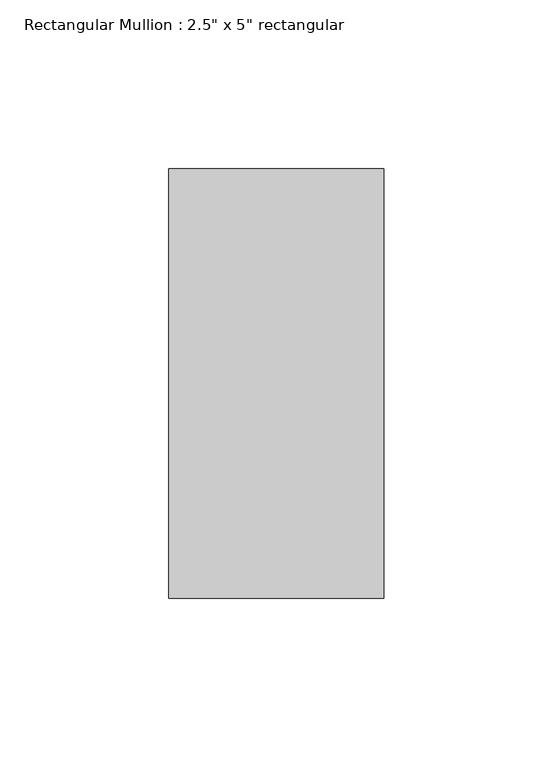
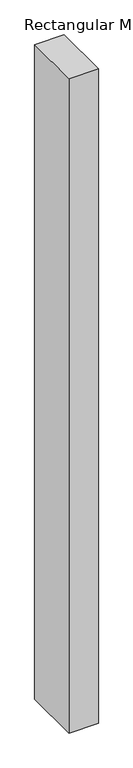
"""IFC4 building model written with IfcOpenShell, lengths in millimetres: member geometry."""

from ifc_helpers import new_model, si_unit, frame, origin, place, context, project, spatial, polyline, outline, extrude, source, transform, mapped, element, save


def member_a27ebcd1(model_context):
    return source(origin(), model_context, "Body", "SweptSolid", [
        extrude(outline(polyline([(31.75, 63.5), (31.75, -63.5), (-31.75, -63.5), (-31.75, 63.5), (31.75, 63.5)])), frame((0.0, 0.0, -1486.7688321), z_axis=(0.0, 0.0, 1.0), x_axis=(1.0, 0.0, 0.0)), (0.0, 0.0, 1.0), 1486.7688321),
    ])


if __name__ == "__main__":
    model = new_model("IFC4")
    model_context = context("Model", 3, world=origin())
    ifc_project = project(units=[si_unit("LENGTHUNIT", "METRE", prefix="MILLI")], contexts=[model_context])
    site = spatial("IfcSite", under=ifc_project)
    building = spatial("IfcBuilding", under=site)
    placement = place(None, origin())
    member_shape = member_a27ebcd1(model_context)
    element("IfcMember", 1, ObjectType="Rectangular Mullion : 2.5\" x 5\" rectangular", at=placement, inside=building, context=model_context, shape_type="MappedRepresentation", body=[
        mapped(member_shape, transform((0.0, 0.0, 0.0), x_axis=(1.0, 0.0, 0.0), y_axis=(0.0, 1.0, 0.0), z_axis=(0.0, 0.0, 1.0))),
    ])
    save(model, "model.ifc")

# Revit data of these elements
# Type "Rectangular Mullion : 2.5\" x 5\" rectangular"
#   built-in parameter 1007304 = 0.416667 (stored number, unit not read)
#   built-in parameter 1007301 = 0.104167 (stored number, unit not read)
#   built-in parameter 1007300 = 0.104167 (stored number, unit not read)
# Element 1 (IfcMember, "Rectangular Mullion : 2.5\" x 5\" rectangular")
#   Materials on its faces: "Aluminum"
# Materials
#   "Aluminum": class "Metal", colour RGB 247 247 247, transparency 0, Description = "Aluminum 6061", Cost = 0
